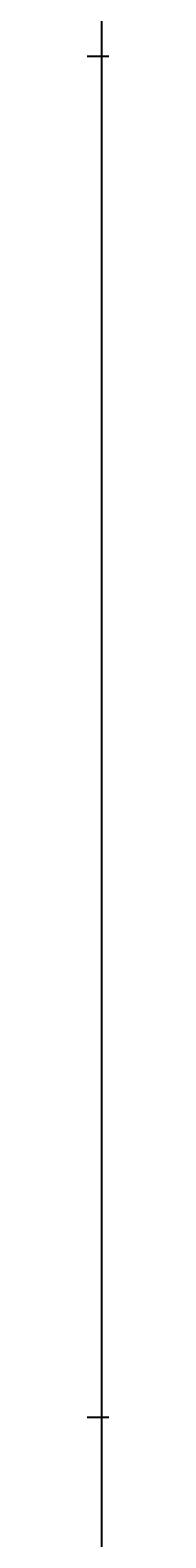
# Model space of a CAD drawing. Units: inches. Extents: x 35362 to 73946, y 43607 to 67532.
# Tile 23 of 134: x 48372 to 48373, y 46091 to 46564. Entities that reach past the tile are written whole.
import ezdxf

# ---------------------------------------------------------------- set-up
doc = ezdxf.new("R2010")
doc.units = ezdxf.units.IN
doc.header["$MEASUREMENT"] = 0
doc.layers.add('A-ANNO-DIMS', color=2, linetype='Continuous', lineweight=18)
doc.styles.get("Standard").update_dxf_attribs({"font": 'arial.ttf'})
doc.dimstyles.get("Standard").update_dxf_attribs({"dimtxt": 0.18, "dimasz": 0.18, "dimexe": 0.18, "dimexo": 0.0625, "dimgap": 0.09, "dimtad": 0, "dimtih": 1, "dimtoh": 1, "dimdec": 4, "dimzin": 0, "dimdsep": 46, "dimtxsty": 'Standard', "dimcen": 0.09, "dimadec": 0, "dimazin": 0, "dimtfac": 1, "dimtdec": 4, "dimtofl": 0, "dimtmove": 0, "dimatfit": 3, "dimfxl": 1, "dimtolj": 1, "dimtzin": 0, "dimarcsym": 0})

# ---------------------------------------------------------------- blocks, each defined once
blk = doc.blocks.new('*D5')
at = {"layer": 'A-ANNO-DIMS', "color": 0, "lineweight": -2, "transparency": 16777216}
for p, q in [((37121.95, 46919.32), (37121.95, 43606.68)), ((69871.5, 45449.83), (69871.5, 43606.68)), ((37122.13, 43606.86), (53496.29, 43606.86)), ((69871.32, 43606.86), (53497.15, 43606.86))]:
    blk.add_line(p, q, dxfattribs=at)
at = {"layer": 'A-ANNO-DIMS', "color": 0, "transparency": 16777216}
for points in [[(37122.13, 43606.89), (37122.13, 43606.83), (37121.95, 43606.86)], [(69871.32, 43606.89), (69871.32, 43606.83), (69871.5, 43606.86)]]:
    blk.add_solid(points, dxfattribs=at)
at = {"layer": 'Defpoints', "color": 0, "transparency": 16777216}
for p in [(37121.95, 46919.38), (69871.5, 45449.89), (69871.5, 43606.86)]:
    blk.add_point(p, dxfattribs=at)
at = {"layer": 'A-ANNO-DIMS', "color": 0, "transparency": 16777216, "insert": (53496.72, 43606.86), "char_height": 0.18, "attachment_point": 5}
blk.add_mtext('\\A1;32750', dxfattribs=at)
blk = doc.blocks.new('*D11')
at = {"layer": 'A-ANNO-DIMS', "color": 0, "lineweight": -2, "transparency": 16777216}
for p, q in [((47978.66, 56028.77), (47978.66, 43606.68)), ((53109.76, 56028.77), (53109.76, 43606.68)), ((47978.84, 43606.86), (50543.87, 43606.86)), ((53109.58, 43606.86), (50544.55, 43606.86))]:
    blk.add_line(p, q, dxfattribs=at)
at = {"layer": 'A-ANNO-DIMS', "color": 0, "transparency": 16777216}
for points in [[(47978.84, 43606.89), (47978.84, 43606.83), (47978.66, 43606.86)], [(53109.58, 43606.89), (53109.58, 43606.83), (53109.76, 43606.86)]]:
    blk.add_solid(points, dxfattribs=at)
at = {"layer": 'Defpoints', "color": 0, "transparency": 16777216}
for p in [(47978.66, 56028.84), (53109.76, 56028.84), (53109.76, 43606.86)]:
    blk.add_point(p, dxfattribs=at)
at = {"layer": 'A-ANNO-DIMS', "color": 0, "transparency": 16777216, "insert": (50544.21, 43606.86), "char_height": 0.18, "attachment_point": 5}
blk.add_mtext('\\A1;5131', dxfattribs=at)
blk = doc.blocks.new('*D27')
at = {"layer": 'A-ANNO-DIMS', "color": 0, "lineweight": -2, "transparency": 16777216}
for p, q in [((47978.66, 56028.77), (47978.66, 43606.68)), ((48373.49, 53428.96), (48373.49, 43606.68)), ((47978.84, 43606.86), (48175.68, 43606.86)), ((48373.31, 43606.86), (48176.47, 43606.86))]:
    blk.add_line(p, q, dxfattribs=at)
at = {"layer": 'A-ANNO-DIMS', "color": 0, "transparency": 16777216}
for points in [[(47978.84, 43606.89), (47978.84, 43606.83), (47978.66, 43606.86)], [(48373.31, 43606.89), (48373.31, 43606.83), (48373.49, 43606.86)]]:
    blk.add_solid(points, dxfattribs=at)
at = {"layer": 'Defpoints', "color": 0, "transparency": 16777216}
for p in [(47978.66, 56028.84), (48373.49, 53429.02), (48373.49, 43606.86)]:
    blk.add_point(p, dxfattribs=at)
at = {"layer": 'A-ANNO-DIMS', "color": 0, "transparency": 16777216, "insert": (48176.08, 43606.86), "char_height": 0.18, "attachment_point": 5}
blk.add_mtext('\\A1;394.8', dxfattribs=at)
blk = doc.blocks.new('*D67')
at = {"layer": 'A-ANNO-DIMS', "color": 0, "lineweight": -2, "transparency": 16777216}
for p, q in [((56873.54, 53351.53), (35361.77, 53351.53)), ((35361.95, 53351.35), (35361.95, 49400.89)), ((35361.95, 45450.07), (35361.95, 49400.53)), ((53793.58, 45449.89), (35361.77, 45449.89))]:
    blk.add_line(p, q, dxfattribs=at)
at = {"layer": 'A-ANNO-DIMS', "color": 0, "transparency": 16777216}
for points in [[(35361.92, 53351.35), (35361.98, 53351.35), (35361.95, 53351.53)], [(35361.92, 45450.07), (35361.98, 45450.07), (35361.95, 45449.89)]]:
    blk.add_solid(points, dxfattribs=at)
at = {"layer": 'Defpoints', "color": 0, "transparency": 16777216}
for p in [(35361.95, 53351.53), (56873.6, 53351.53), (53793.64, 45449.89)]:
    blk.add_point(p, dxfattribs=at)
at = {"layer": 'A-ANNO-DIMS', "color": 0, "transparency": 16777216, "insert": (35361.95, 49400.71), "char_height": 0.18, "attachment_point": 5}
blk.add_mtext('\\A1;7901.6', dxfattribs=at)
blk = doc.blocks.new('*D76')
at = {"layer": 'A-ANNO-DIMS', "color": 0, "lineweight": -2, "transparency": 16777216}
for p, q in [((54052.84, 46555.29), (35361.77, 46555.29)), ((35361.95, 46555.11), (35361.95, 46342.27)), ((35361.95, 46129.06), (35361.95, 46341.9)), ((53793.58, 46128.88), (35361.77, 46128.88))]:
    blk.add_line(p, q, dxfattribs=at)
at = {"layer": 'A-ANNO-DIMS', "color": 0, "transparency": 16777216}
for points in [[(35361.92, 46555.11), (35361.98, 46555.11), (35361.95, 46555.29)], [(35361.92, 46129.06), (35361.98, 46129.06), (35361.95, 46128.88)]]:
    blk.add_solid(points, dxfattribs=at)
at = {"layer": 'Defpoints', "color": 0, "transparency": 16777216}
for p in [(35361.95, 46555.29), (54052.9, 46555.29), (53793.64, 46128.88)]:
    blk.add_point(p, dxfattribs=at)
at = {"layer": 'A-ANNO-DIMS', "color": 0, "transparency": 16777216, "insert": (35361.95, 46342.09), "char_height": 0.18, "attachment_point": 5}
blk.add_mtext('\\A1;426.4', dxfattribs=at)
blk = doc.blocks.new('*D90')
at = {"layer": 'A-ANNO-DIMS', "color": 0, "lineweight": -2, "transparency": 16777216}
for p, q in [((53707.72, 47291.29), (35361.77, 47291.29)), ((35361.95, 47291.11), (35361.95, 46710.26)), ((35361.95, 46129.06), (35361.95, 46709.9)), ((53793.58, 46128.88), (35361.77, 46128.88))]:
    blk.add_line(p, q, dxfattribs=at)
at = {"layer": 'A-ANNO-DIMS', "color": 0, "transparency": 16777216}
for points in [[(35361.92, 47291.11), (35361.98, 47291.11), (35361.95, 47291.29)], [(35361.92, 46129.06), (35361.98, 46129.06), (35361.95, 46128.88)]]:
    blk.add_solid(points, dxfattribs=at)
at = {"layer": 'Defpoints', "color": 0, "transparency": 16777216}
for p in [(53707.78, 47291.29), (35361.95, 46128.88), (53793.64, 46128.88)]:
    blk.add_point(p, dxfattribs=at)
at = {"layer": 'A-ANNO-DIMS', "color": 0, "transparency": 16777216, "insert": (35361.95, 46710.08), "char_height": 0.18, "attachment_point": 5}
blk.add_mtext('\\A1;1162.4', dxfattribs=at)

msp = doc.modelspace()

# ---------------------------------------------------------------- dimensions: what is measured, and where the dimension line sits
at = {"layer": 'A-ANNO-DIMS'}
for base, p1, p2, override, picture, middle in [((53109.76, 43606.859), (47978.665, 56028.836), (53109.76, 56028.836), {"dimdec": 0, "dimlfac": 1, "dimrnd": 0, "dimzin": 0, "dimdsep": 46, "dimlunit": 2}, '*D11', (50544.212, 43606.859)), ((48373.492, 43606.859), (47978.665, 56028.836), (48373.492, 53429.019), {"dimdec": 1, "dimlfac": 1, "dimrnd": 0, "dimzin": 0, "dimdsep": 46, "dimlunit": 2}, '*D27', (48176.078, 43606.859)), ((69871.496, 43606.859), (37121.949, 46919.381), (69871.496, 45449.894), {"dimdec": 0, "dimlfac": 1, "dimrnd": 0, "dimzin": 0, "dimdsep": 46, "dimlunit": 2}, '*D5', (53496.723, 43606.859))]:
    dim = msp.add_linear_dim(base=base, p1=p1, p2=p2, dimstyle='Standard', override=override, dxfattribs=at)
    dim.commit()
    dim.dimension.update_dxf_attribs({"geometry": picture, "text_midpoint": middle})
for base, p1, p2, picture, middle in [((35361.949, 53351.529), (53793.638, 45449.894), (56873.602, 53351.529), '*D67', (35361.949, 49400.712)), ((35361.949, 46128.878), (53707.781, 47291.285), (53793.638, 46128.878), '*D90', (35361.949, 46710.081)), ((35361.949, 46555.293), (53793.638, 46128.878), (54052.899, 46555.293), '*D76', (35361.949, 46342.086))]:
    dim = msp.add_linear_dim(base=base, p1=p1, p2=p2, angle=90, dimstyle='Standard', override={"dimdec": 1, "dimlfac": 1, "dimrnd": 0, "dimzin": 0, "dimdsep": 46, "dimlunit": 2}, dxfattribs=at)
    dim.commit()
    dim.dimension.update_dxf_attribs({"geometry": picture, "text_midpoint": middle})

doc.saveas('drawing.dxf')
